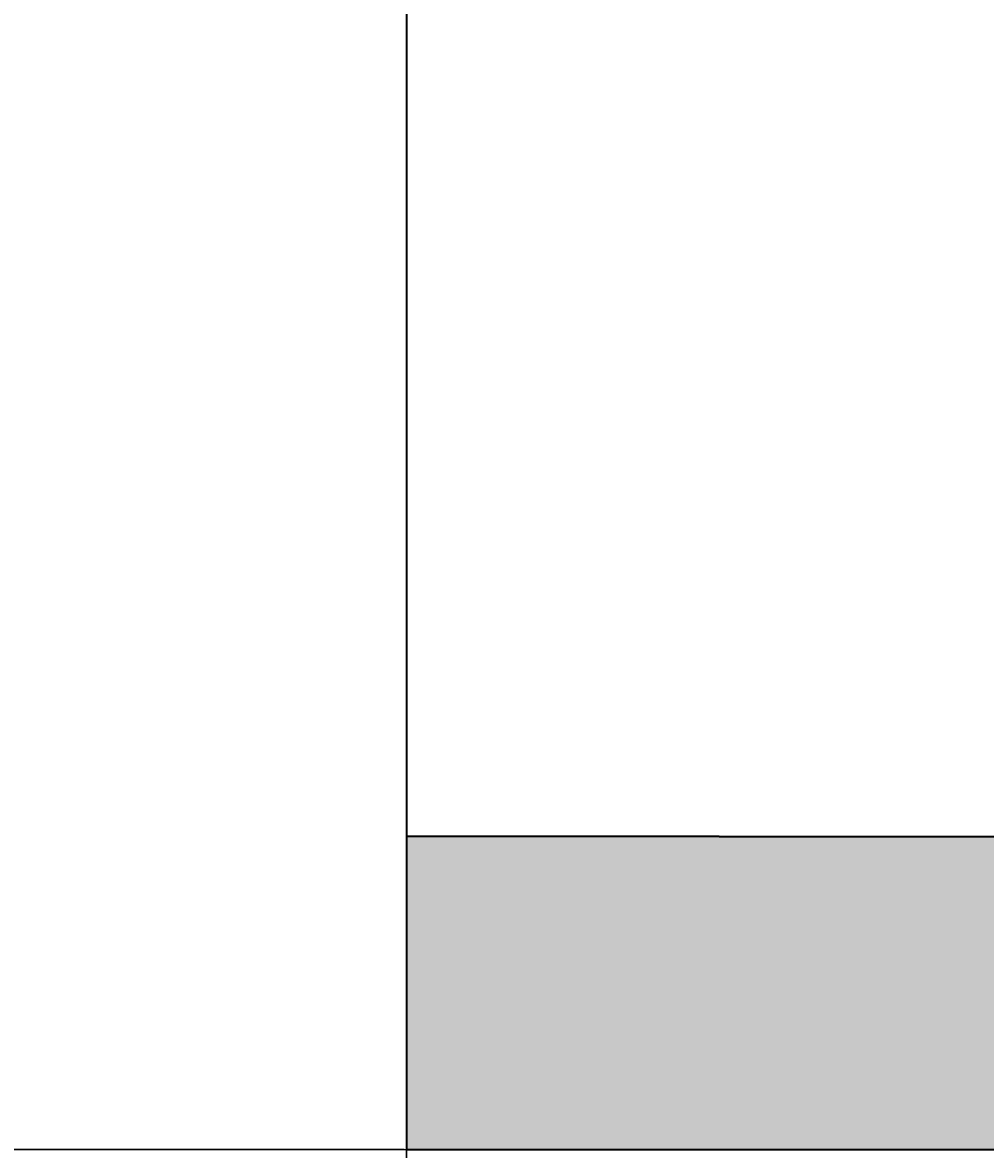
# Model space of a CAD drawing. Units: inches. Extents: x 1998 to 2588, y 1139 to 1977.
# Tile 99 of 134: x 2397 to 2425, y 1523 to 1555. Entities that reach past the tile are written whole.
import ezdxf

# ---------------------------------------------------------------- set-up
doc = ezdxf.new("R2010")
doc.units = ezdxf.units.IN
for name, color, linetype, lineweight in [('A-ANNO-DIMS', 2, 'Continuous', 18), ('A-FLOR-EVTR', 7, 'Continuous', 35), ('A-FLOR-STRS', 7, 'Continuous', 25), ('A-WALL-PATT', 252, 'Continuous', 13)]:
    doc.layers.add(name, color=color, linetype=linetype, lineweight=lineweight)
doc.styles.get("Standard").update_dxf_attribs({"font": 'arial.ttf'})
doc.dimstyles.get("Standard").update_dxf_attribs({"dimtxt": 0.18, "dimasz": 0.18, "dimexe": 0.18, "dimexo": 0.0625, "dimgap": 0.09, "dimtad": 0, "dimtih": 1, "dimtoh": 1, "dimdec": 4, "dimzin": 0, "dimdsep": 46, "dimtxsty": 'Standard', "dimcen": 0.09, "dimadec": 0, "dimazin": 0, "dimtfac": 1, "dimtdec": 4, "dimtofl": 0, "dimtmove": 0, "dimatfit": 3, "dimfxl": 1, "dimtolj": 1, "dimtzin": 0, "dimarcsym": 0})

# ---------------------------------------------------------------- blocks, each defined once
blk = doc.blocks.new('*D24')
at = {"layer": 'A-ANNO-DIMS', "color": 0, "lineweight": -2, "transparency": 16777216}
for p, q in [((2398.535, 1911.232), (2588.309, 1911.232)), ((2588.129, 1911.052), (2588.129, 1570.164)), ((2588.129, 1228.912), (2588.129, 1569.8)), ((2527.535, 1228.732), (2588.309, 1228.732))]:
    blk.add_line(p, q, dxfattribs=at)
at = {"layer": 'A-ANNO-DIMS', "color": 0, "transparency": 16777216}
for points in [[(2588.099, 1911.052), (2588.159, 1911.052), (2588.129, 1911.232)], [(2588.099, 1228.912), (2588.159, 1228.912), (2588.129, 1228.732)]]:
    blk.add_solid(points, dxfattribs=at)
at = {"layer": 'Defpoints', "color": 0, "transparency": 16777216}
for p in [(2398.473, 1911.232), (2588.129, 1911.232), (2527.473, 1228.732)]:
    blk.add_point(p, dxfattribs=at)
at = {"layer": 'A-ANNO-DIMS', "color": 0, "transparency": 16777216, "insert": (2588.129, 1569.982), "char_height": 0.18, "attachment_point": 5}
blk.add_mtext('\\A1;682.5', dxfattribs=at)
blk = doc.blocks.new('*D34')
at = {"layer": 'A-ANNO-DIMS', "color": 0, "lineweight": -2, "transparency": 16777216}
for p, q in [((2407.91, 1594.732), (1997.843, 1594.732)), ((1998.023, 1594.552), (1998.023, 1558.913)), ((1998.023, 1522.912), (1998.023, 1558.552)), ((2407.91, 1522.732), (1997.843, 1522.732))]:
    blk.add_line(p, q, dxfattribs=at)
at = {"layer": 'A-ANNO-DIMS', "color": 0, "transparency": 16777216}
for points in [[(1997.993, 1594.552), (1998.053, 1594.552), (1998.023, 1594.732)], [(1997.993, 1522.912), (1998.053, 1522.912), (1998.023, 1522.732)]]:
    blk.add_solid(points, dxfattribs=at)
at = {"layer": 'Defpoints', "color": 0, "transparency": 16777216}
for p in [(1998.023, 1594.732), (2407.973, 1594.732), (2407.973, 1522.732)]:
    blk.add_point(p, dxfattribs=at)
at = {"layer": 'A-ANNO-DIMS', "color": 0, "transparency": 16777216, "insert": (1998.023, 1558.732), "char_height": 0.18, "attachment_point": 5}
blk.add_mtext('\\A1;72', dxfattribs=at)
blk = doc.blocks.new('*D42')
at = {"layer": 'A-ANNO-DIMS', "color": 0, "lineweight": -2, "transparency": 16777216}
for p, q in [((2287.535, 1588.732), (2588.309, 1588.732)), ((2588.129, 1588.552), (2588.129, 1555.914)), ((2588.129, 1522.912), (2588.129, 1555.55)), ((2287.535, 1522.732), (2588.309, 1522.732))]:
    blk.add_line(p, q, dxfattribs=at)
at = {"layer": 'A-ANNO-DIMS', "color": 0, "transparency": 16777216}
for points in [[(2588.099, 1588.552), (2588.159, 1588.552), (2588.129, 1588.732)], [(2588.099, 1522.912), (2588.159, 1522.912), (2588.129, 1522.732)]]:
    blk.add_solid(points, dxfattribs=at)
at = {"layer": 'Defpoints', "color": 0, "transparency": 16777216}
for p in [(2287.473, 1588.732), (2588.129, 1588.732), (2287.473, 1522.732)]:
    blk.add_point(p, dxfattribs=at)
at = {"layer": 'A-ANNO-DIMS', "color": 0, "transparency": 16777216, "insert": (2588.129, 1555.732), "char_height": 0.18, "attachment_point": 5}
blk.add_mtext('\\A1;66', dxfattribs=at)
blk = doc.blocks.new('*D43')
at = {"layer": 'A-ANNO-DIMS', "color": 0, "lineweight": -2, "transparency": 16777216}
for p, q in [((2407.973, 1594.67), (2407.973, 1138.602)), ((2345.973, 1588.67), (2345.973, 1138.602)), ((2346.153, 1138.782), (2376.754, 1138.782)), ((2407.793, 1138.782), (2377.191, 1138.782))]:
    blk.add_line(p, q, dxfattribs=at)
at = {"layer": 'A-ANNO-DIMS', "color": 0, "transparency": 16777216}
for points in [[(2346.153, 1138.812), (2346.153, 1138.752), (2345.973, 1138.782)], [(2407.793, 1138.812), (2407.793, 1138.752), (2407.973, 1138.782)]]:
    blk.add_solid(points, dxfattribs=at)
at = {"layer": 'Defpoints', "color": 0, "transparency": 16777216}
for p in [(2407.973, 1594.732), (2345.973, 1588.732), (2407.973, 1138.782)]:
    blk.add_point(p, dxfattribs=at)
at = {"layer": 'A-ANNO-DIMS', "color": 0, "transparency": 16777216, "insert": (2376.973, 1138.782), "char_height": 0.18, "attachment_point": 5}
blk.add_mtext('\\A1;62', dxfattribs=at)

msp = doc.modelspace()

# ---------------------------------------------------------------- hatches: boundary and pattern name
at = {"layer": 'A-WALL-PATT'}
h = msp.add_hatch(color=256, dxfattribs=at)
h.dxf.hatch_style = 1
h.paths.add_polyline_path([(2527.4729, 1362.2324), (2510.9729, 1362.2324), (2510.9729, 1357.7324), (2518.4729, 1357.7324), (2518.4729, 1237.7324), (2503.1458, 1237.7324), (2503.1458, 1228.7324), (2527.4729, 1228.7324)])
h.paths.add_polyline_path([(2490.5682, 1362.2324), (2398.4729, 1362.2324), (2398.4729, 1357.7324), (2490.5682, 1357.7324)])
h.paths.add_polyline_path([(2224.9729, 1264.7324), (2222.9729, 1264.7324), (2222.9729, 1232.4125), (2341.4729, 1232.4125), (2341.4729, 1234.4125), (2224.9729, 1234.4125)])
h.paths.add_polyline_path([(2334.5332, 1273.7324), (2264.7638, 1273.7324), (2264.7638, 1269.5611, -0.043659), (2264.3413, 1264.7324), (2334.5332, 1264.7324)])
h.paths.add_polyline_path([(2236.9551, 1273.7324), (2234.4125, 1273.7324), (2234.4125, 1264.7324), (2236.9551, 1264.7324), (2236.9551, 1269.5611)])
h.paths.add_polyline_path([(2222.9729, 1293.2324), (2096.9729, 1293.2324), (2096.9729, 1345.0966), (2087.9729, 1345.0966), (2087.9729, 1284.2324), (2222.9729, 1284.2324), (2222.9729, 1285.137)])
h.paths.add_polyline_path([(2096.9729, 1458.7927), (2087.9729, 1458.7927), (2087.9729, 1417.7324), (2087.9729, 1413.2324), (2096.9729, 1413.2324), (2096.9729, 1417.7324)])
h.paths.add_polyline_path([(2096.9729, 1413.2324), (2087.9729, 1413.2324), (2087.9729, 1365.5012), (2096.9729, 1365.5012), (2096.9729, 1369.3358)])
h.paths.add_polyline_path([(2186.2943, 1417.7324), (2138.6074, 1417.7324), (2096.9729, 1417.7324), (2096.9729, 1413.2324), (2138.6074, 1413.2324), (2186.2943, 1413.2324)])
h.paths.add_polyline_path([(2181.4729, 1465.7324), (2176.9729, 1465.7324), (2176.9729, 1451.6434), (2181.4729, 1451.6434)])
h.paths.add_polyline_path([(2181.4729, 1422.1664), (2176.9729, 1422.1664), (2176.9729, 1417.7324), (2181.4729, 1417.7324)])
h.paths.add_polyline_path([(2063.9729, 1465.7324), (2087.9729, 1465.7324), (2087.9729, 1470.2324), (2059.4729, 1470.2324), (2059.4729, 1413.2324), (2087.9729, 1413.2324), (2087.9729, 1417.7324), (2063.9729, 1417.7324)])
h.paths.add_polyline_path([(2181.4729, 1755.2324), (2176.9729, 1755.2324), (2176.9729, 1748.6798), (2177.0513, 1748.6798), (2181.4729, 1748.6798)])
h.paths.add_polyline_path([(2227.4729, 1707.2324), (2220.4647, 1707.2324), (2220.4647, 1702.7324), (2222.9729, 1702.7324), (2222.9729, 1604.637), (2227.4729, 1604.637)])
h.paths.add_polyline_path([(2114.9729, 1702.7324), (2105.9729, 1702.7324), (2105.9729, 1628.4781, -0.0318759), (2110.1012, 1628.7416), (2114.9729, 1628.7416)])
h.paths.add_polyline_path([(2345.9729, 1739.3278), (2341.4729, 1739.3278), (2341.4729, 1647.5211), (2345.9729, 1647.5211)])
h.paths.add_polyline_path([(2350.6273, 1641.2324), (2345.9729, 1641.2324), (2345.9729, 1636.7324), (2350.6273, 1636.7324), (2350.6273, 1639.8729)])
h.paths.add_polyline_path([(2501.9729, 1641.2324), (2407.9729, 1641.2324), (2392.5005, 1641.2324), (2392.5005, 1639.8729), (2392.5005, 1636.7324), (2501.9729, 1636.7324)])
h.paths.add_polyline_path([(2510.9729, 1755.2324), (2501.9729, 1755.2324), (2501.9729, 1641.2324), (2510.9729, 1641.2324)])
h.paths.add_polyline_path([(2549.1786, 1641.2324), (2522.3775, 1641.2324), (2522.3775, 1636.7324), (2540.1786, 1636.7324), (2540.1786, 1480.7324), (2522.3775, 1480.7324), (2522.3775, 1476.2324), (2549.1786, 1476.2324)])
h.paths.add_polyline_path([(2498.1786, 1594.7324), (2407.9729, 1594.7324), (2407.9729, 1585.7324), (2416.9729, 1585.7324), (2489.1786, 1585.7324), (2489.1786, 1531.7324), (2416.9729, 1531.7324), (2407.9729, 1531.7324), (2407.9729, 1522.7324), (2498.1786, 1522.7324)])
h.paths.add_polyline_path([(2351.6437, 1480.7324), (2345.9729, 1480.7324), (2345.9729, 1476.2324), (2351.6437, 1476.2324), (2351.6437, 1477.5919)])
h.paths.add_polyline_path([(2501.9729, 1480.7324), (2498.1786, 1480.7324), (2407.9729, 1480.7324), (2393.5168, 1480.7324), (2393.5168, 1477.5919), (2393.5168, 1476.2324), (2501.9729, 1476.2324)])

# ---------------------------------------------------------------- linework, layer by layer
at = {"layer": 'A-FLOR-EVTR'}
msp.add_line((2416.9729, 1531.7324), (2407.9729, 1531.7324), dxfattribs=at)
msp.add_lwpolyline([(2407.9729, 1522.7324), (2498.1786, 1522.7324), (2498.1786, 1594.7324), (2407.9729, 1594.7324)], close=True, dxfattribs=at)
msp.add_lwpolyline([(2416.9729, 1531.7324), (2489.1786, 1531.7324), (2489.1786, 1585.7324), (2416.9729, 1585.7324)], dxfattribs=at)
at = {"layer": 'A-FLOR-STRS'}
msp.add_line((2407.9729, 1480.7324), (2407.9729, 1636.7324), dxfattribs=at)

# ---------------------------------------------------------------- dimensions: what is measured, and where the dimension line sits
at = {"layer": 'A-ANNO-DIMS'}
for base, p1, p2, override, picture, middle in [((2588.1286, 1911.2324), (2527.4729, 1228.7324), (2398.4729, 1911.2324), {"dimdec": 1, "dimlfac": 1, "dimrnd": 0, "dimzin": 0, "dimdsep": 46, "dimlunit": 2}, '*D24', (2588.1286, 1569.9824)), ((1998.0229, 1594.7324), (2407.9729, 1522.7324), (2407.9729, 1594.7324), {"dimdec": 0, "dimlfac": 1, "dimrnd": 0, "dimzin": 0, "dimdsep": 46, "dimlunit": 2}, '*D34', (1998.0229, 1558.7324)), ((2588.1286, 1588.7324), (2287.4729, 1522.7324), (2287.4729, 1588.7324), {"dimdec": 0, "dimlfac": 1, "dimrnd": 0, "dimzin": 0, "dimdsep": 46, "dimlunit": 2}, '*D42', (2588.1286, 1555.7324))]:
    dim = msp.add_linear_dim(base=base, p1=p1, p2=p2, angle=90, dimstyle='Standard', override=override, dxfattribs=at)
    dim.commit()
    dim.dimension.update_dxf_attribs({"geometry": picture, "text_midpoint": middle})
dim = msp.add_linear_dim(base=(2407.9729, 1138.7824), p1=(2345.9729, 1588.7324), p2=(2407.9729, 1594.7324), dimstyle='Standard', override={"dimdec": 0, "dimlfac": 1, "dimrnd": 0, "dimzin": 0, "dimdsep": 46, "dimlunit": 2}, dxfattribs=at)
dim.commit()
dim.dimension.update_dxf_attribs({"geometry": '*D43', "text_midpoint": (2376.9729, 1138.7824)})

doc.saveas('drawing.dxf')
